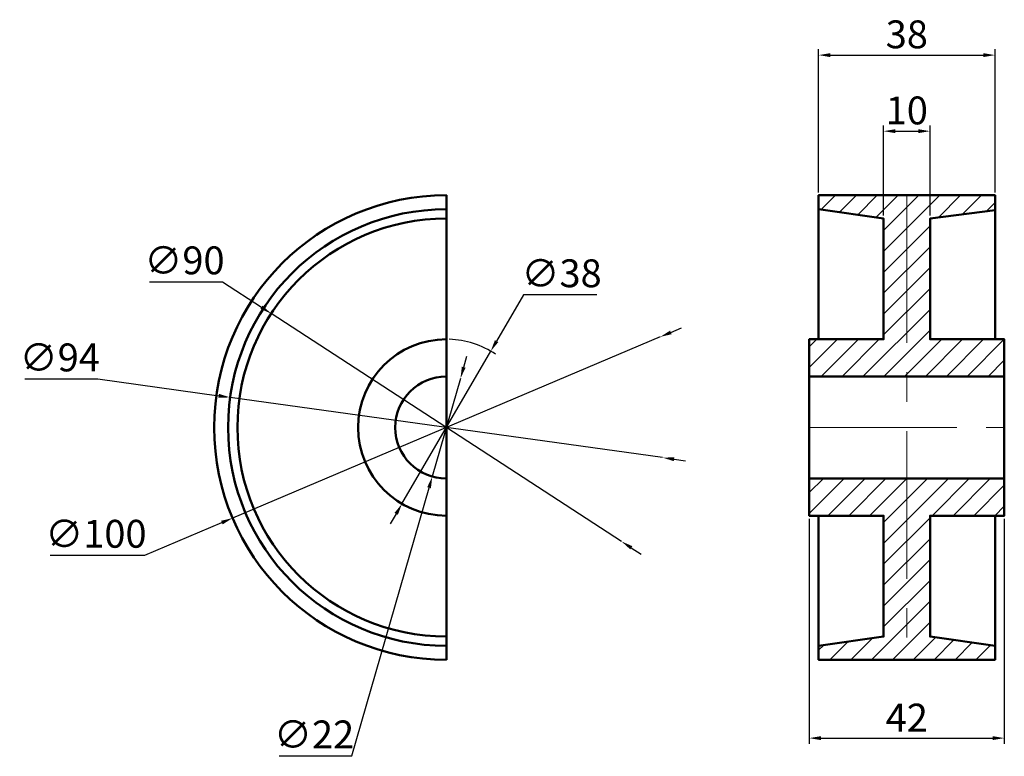
# Model space of a CAD drawing. Units: millimetres. Extents: x 59 to 271, y 50 to 208.
import ezdxf

# ---------------------------------------------------------------- set-up
doc = ezdxf.new("R2010")
doc.units = ezdxf.units.MM
doc.linetypes.add('CENTER', pattern=[50.8, 31.75, -6.35, 6.35, -6.35])
for name, color, linetype, lineweight in [('M-CNTR', 1, 'CENTER', 18), ('M-DIMS', 2, 'Continuous', 25), ('M-HATC', 8, 'Continuous', 18), ('M-OUTL', 7, 'Continuous', 50)]:
    doc.layers.add(name, color=color, linetype=linetype, lineweight=lineweight)
doc.styles.get("Standard").update_dxf_attribs({"font": 'arial.ttf'})
doc.dimstyles.new('ISO-25', dxfattribs={"dimtxt": 6, "dimasz": 2.5, "dimexe": 1.25, "dimexo": 0.625, "dimtad": 1, "dimtoh": 1, "dimdec": 0, "dimtxsty": 'Standard', "dimcen": 2.5, "dimadec": 0, "dimazin": 0, "dimtfac": 1, "dimtdec": 0, "dimtmove": 0, "dimatfit": 3, "dimfxl": 1, "dimarcsym": 0})

# ---------------------------------------------------------------- blocks, each defined once
blk = doc.blocks.new('*D1')
at = {"layer": 'Defpoints', "color": 0, "transparency": 16777216}
for p in [(255.48, 184.43), (245.48, 165.63), (255.48, 165.63)]:
    blk.add_point(p, dxfattribs=at)
at = {"layer": 'M-DIMS', "color": 0, "lineweight": -2, "transparency": 16777216}
for p, q in [((245.48, 166.25), (245.48, 185.68)), ((255.48, 166.25), (255.48, 185.68)), ((247.98, 184.43), (252.98, 184.43))]:
    blk.add_line(p, q, dxfattribs=at)
at = {"layer": 'M-DIMS', "color": 0, "transparency": 16777216}
for points in [[(247.98, 184.85), (247.98, 184.02), (245.48, 184.43)], [(252.98, 184.85), (252.98, 184.02), (255.48, 184.43)]]:
    blk.add_solid(points, dxfattribs=at)
at = {"layer": 'M-DIMS', "color": 0, "transparency": 16777216, "insert": (250.48, 188.12), "char_height": 6, "attachment_point": 5}
blk.add_mtext('10', dxfattribs=at)
blk = doc.blocks.new('*D2')
at = {"layer": 'Defpoints', "color": 0, "transparency": 16777216}
for p in [(269.48, 200.81), (231.48, 170.63), (269.48, 170.63)]:
    blk.add_point(p, dxfattribs=at)
at = {"layer": 'M-DIMS', "color": 0, "lineweight": -2, "transparency": 16777216}
for p, q in [((231.48, 171.25), (231.48, 202.06)), ((269.48, 171.25), (269.48, 202.06)), ((233.98, 200.81), (266.98, 200.81))]:
    blk.add_line(p, q, dxfattribs=at)
at = {"layer": 'M-DIMS', "color": 0, "transparency": 16777216}
for points in [[(233.98, 201.22), (233.98, 200.39), (231.48, 200.81)], [(266.98, 201.22), (266.98, 200.39), (269.48, 200.81)]]:
    blk.add_solid(points, dxfattribs=at)
at = {"layer": 'M-DIMS', "color": 0, "transparency": 16777216, "insert": (250.48, 204.5), "char_height": 6, "attachment_point": 5}
blk.add_mtext('38', dxfattribs=at)
blk = doc.blocks.new('*D3')
at = {"layer": 'Defpoints', "color": 0, "transparency": 16777216}
for p in [(229.48, 101.63), (271.48, 101.63), (271.48, 53.75)]:
    blk.add_point(p, dxfattribs=at)
at = {"layer": 'M-DIMS', "color": 0, "lineweight": -2, "transparency": 16777216}
for p, q in [((229.48, 101), (229.48, 52.5)), ((271.48, 101), (271.48, 52.5)), ((231.98, 53.75), (268.98, 53.75))]:
    blk.add_line(p, q, dxfattribs=at)
at = {"layer": 'M-DIMS', "color": 0, "transparency": 16777216}
for points in [[(231.98, 54.17), (231.98, 53.33), (229.48, 53.75)], [(268.98, 54.17), (268.98, 53.33), (271.48, 53.75)]]:
    blk.add_solid(points, dxfattribs=at)
at = {"layer": 'M-DIMS', "color": 0, "transparency": 16777216, "insert": (250.48, 57.39), "char_height": 6, "attachment_point": 5}
blk.add_mtext('42', dxfattribs=at)
blk = doc.blocks.new('*D4')
at = {"layer": 'Defpoints', "color": 0, "transparency": 16777216}
for p in [(197.37, 140.13), (105.29, 101.13)]:
    blk.add_point(p, dxfattribs=at)
at = {"layer": 'M-DIMS', "color": 0, "lineweight": -2, "transparency": 16777216}
for p, q in [((199.67, 141.1), (201.97, 142.08)), ((197.37, 140.13), (105.29, 101.13)), ((86.37, 93.11), (102.99, 100.15)), ((65.98, 93.11), (86.37, 93.11))]:
    blk.add_line(p, q, dxfattribs=at)
at = {"layer": 'M-DIMS', "color": 0, "transparency": 16777216}
for points in [[(199.51, 141.49), (199.83, 140.72), (197.37, 140.13)], [(102.82, 100.54), (103.15, 99.77), (105.29, 101.13)]]:
    blk.add_solid(points, dxfattribs=at)
at = {"layer": 'M-DIMS', "color": 0, "transparency": 16777216, "insert": (75.86, 96.97), "char_height": 6, "attachment_point": 5}
blk.add_mtext('∅100', dxfattribs=at)
blk = doc.blocks.new('*D5')
at = {"layer": 'Defpoints', "color": 0, "transparency": 16777216}
for p in [(104.78, 127.11), (197.88, 114.14)]:
    blk.add_point(p, dxfattribs=at)
at = {"layer": 'M-DIMS', "color": 0, "lineweight": -2, "transparency": 16777216}
for p, q in [((60.53, 131.08), (76.26, 131.08)), ((76.26, 131.08), (102.3, 127.46)), ((197.88, 114.14), (104.78, 127.11)), ((200.35, 113.8), (202.83, 113.45))]:
    blk.add_line(p, q, dxfattribs=at)
at = {"layer": 'M-DIMS', "color": 0, "transparency": 16777216}
for points in [[(102.36, 127.87), (102.24, 127.04), (104.78, 127.11)], [(200.41, 114.21), (200.3, 113.39), (197.88, 114.14)]]:
    blk.add_solid(points, dxfattribs=at)
at = {"layer": 'M-DIMS', "color": 0, "transparency": 16777216, "insert": (68.08, 134.94), "char_height": 6, "attachment_point": 5}
blk.add_mtext('∅94', dxfattribs=at)
blk = doc.blocks.new('*D6')
at = {"layer": 'Defpoints', "color": 0, "transparency": 16777216}
for p in [(113.6, 145.16), (189.05, 96.1)]:
    blk.add_point(p, dxfattribs=at)
at = {"layer": 'M-DIMS', "color": 0, "lineweight": -2, "transparency": 16777216}
for p, q in [((87.37, 151.99), (103.1, 151.99)), ((103.1, 151.99), (111.51, 146.52)), ((189.05, 96.1), (113.6, 145.16)), ((191.15, 94.73), (193.25, 93.37))]:
    blk.add_line(p, q, dxfattribs=at)
at = {"layer": 'M-DIMS', "color": 0, "transparency": 16777216}
for points in [[(111.73, 146.87), (111.28, 146.17), (113.6, 145.16)], [(191.38, 95.08), (190.92, 94.39), (189.05, 96.1)]]:
    blk.add_solid(points, dxfattribs=at)
at = {"layer": 'M-DIMS', "color": 0, "transparency": 16777216, "insert": (94.93, 155.84), "char_height": 6, "attachment_point": 5}
blk.add_mtext('∅90', dxfattribs=at)
blk = doc.blocks.new('*D7')
at = {"layer": 'Defpoints', "color": 0, "transparency": 16777216}
for p in [(160.88, 137.05), (141.77, 104.2)]:
    blk.add_point(p, dxfattribs=at)
at = {"layer": 'M-DIMS', "color": 0, "lineweight": -2, "transparency": 16777216}
for p, q in [((167.95, 149.2), (162.14, 139.21)), ((183.71, 149.2), (167.95, 149.2)), ((141.77, 104.2), (160.88, 137.05)), ((140.52, 102.04), (139.26, 99.88))]:
    blk.add_line(p, q, dxfattribs=at)
blk.add_arc((151.33, 120.63), 19, 56.0417, 88.1153, dxfattribs=at)
at = {"layer": 'M-DIMS', "color": 0, "transparency": 16777216}
for points in [[(161.78, 139.42), (162.5, 139), (160.88, 137.05)], [(140.16, 102.25), (140.88, 101.83), (141.77, 104.2)]]:
    blk.add_solid(points, dxfattribs=at)
at = {"layer": 'M-DIMS', "color": 0, "transparency": 16777216, "insert": (176.14, 153.06), "char_height": 6, "attachment_point": 5}
blk.add_mtext('∅38', dxfattribs=at)
blk = doc.blocks.new('*D8')
at = {"layer": 'Defpoints', "color": 0, "transparency": 16777216}
for p in [(154.37, 131.2), (148.29, 110.06)]:
    blk.add_point(p, dxfattribs=at)
at = {"layer": 'M-DIMS', "color": 0, "lineweight": -2, "transparency": 16777216}
for p, q in [((155.06, 133.6), (155.75, 136)), ((154.37, 131.2), (148.29, 110.06)), ((130.99, 49.92), (147.6, 107.65)), ((115.31, 49.92), (130.99, 49.92))]:
    blk.add_line(p, q, dxfattribs=at)
at = {"layer": 'M-DIMS', "color": 0, "transparency": 16777216}
for points in [[(154.66, 133.72), (155.46, 133.49), (154.37, 131.2)], [(147.2, 107.77), (148, 107.54), (148.29, 110.06)]]:
    blk.add_solid(points, dxfattribs=at)
at = {"layer": 'M-DIMS', "color": 0, "transparency": 16777216, "insert": (122.84, 53.77), "char_height": 6, "attachment_point": 5}
blk.add_mtext('∅22', dxfattribs=at)

msp = doc.modelspace()

# ---------------------------------------------------------------- hatches: boundary and pattern name
at = {"layer": 'M-HATC'}
h = msp.add_hatch(dxfattribs=at)
h.set_pattern_fill('ANSI31', color=256)
h.set_pattern_definition([(45, (60.016, 0), (-2.245064, 2.245064), [])])
h.paths.add_polyline_path([(250.48, 170.63), (231.48, 170.63), (231.48, 167.63), (245.48, 165.63), (245.48, 139.63), (231.48, 139.63), (229.48, 139.63), (229.48, 131.63), (250.48, 131.63)])
h.paths.add_polyline_path([(271.48, 139.63), (269.48, 139.63), (255.48, 139.63), (255.48, 165.63), (269.48, 167.45), (269.48, 170.63), (250.48, 170.63), (250.48, 131.63), (271.48, 131.63)])
h.paths.add_polyline_path([(271.48, 109.63), (250.48, 109.63), (250.48, 70.63), (269.48, 70.63), (269.48, 73.63), (255.48, 75.63), (255.48, 101.63), (269.48, 101.63), (271.48, 101.63)])
h.paths.add_polyline_path([(250.48, 109.63), (229.48, 109.63), (229.48, 101.63), (231.48, 101.63), (245.48, 101.63), (245.48, 75.63), (231.48, 73.63), (231.48, 70.63), (250.48, 70.63)])

# ---------------------------------------------------------------- linework, layer by layer
at = {"layer": 'M-CNTR'}
for p, q in [((250.48, 170.63), (250.48, 70.63)), ((229.48, 120.63), (271.48, 120.63))]:
    msp.add_line(p, q, dxfattribs=at)
at = {"layer": 'M-OUTL'}
for p, q in [((271.48, 131.63), (229.48, 131.63)), ((229.48, 109.63), (271.48, 109.63))]:
    msp.add_line(p, q, dxfattribs=at)
msp.add_lwpolyline([(151.33, 70.63), (151.33, 170.63, 1)], format="xyb", close=True, dxfattribs=at)
for points in [[(231.48, 139.63), (231.48, 170.63), (269.48, 170.63), (269.48, 139.63)], [(269.48, 73.63), (255.48, 75.63), (255.48, 101.63), (269.48, 101.63), (269.48, 70.63), (231.48, 70.63), (231.48, 101.63), (229.48, 101.63), (229.48, 139.63), (231.48, 139.63), (245.48, 139.63), (245.48, 165.63), (231.48, 167.63)], [(269.48, 101.63), (271.48, 101.63), (271.48, 139.63), (269.48, 139.63), (255.48, 139.63), (255.48, 165.63), (269.48, 167.45)], [(231.48, 73.63), (245.48, 75.63), (245.48, 101.63), (231.48, 101.63)]]:
    msp.add_lwpolyline(points, dxfattribs=at)
for radius in [47, 45, 19, 11]:
    msp.add_arc((151.33, 120.63), radius, 90, 270, dxfattribs=at)

# ---------------------------------------------------------------- dimensions: what is measured, and where the dimension line sits
at = {"layer": 'M-DIMS'}
for base, p1, p2, picture, middle in [((269.48, 200.81), (231.48, 170.63), (269.48, 170.63), '*D2', (250.48, 204.5)), ((255.48, 184.43), (245.48, 165.63), (255.48, 165.63), '*D1', (250.48, 188.12)), ((271.48, 53.75), (229.48, 101.63), (271.48, 101.63), '*D3', (250.48, 57.39))]:
    dim = msp.add_linear_dim(base=base, p1=p1, p2=p2, dimstyle='ISO-25', override={"dimclrd": 0, "dimclre": 0, "dimclrt": 0}, dxfattribs=at)
    dim.commit()
    dim.dimension.update_dxf_attribs({"geometry": picture, "text_midpoint": middle})
for p1, p2, picture, middle in [((189.05, 96.1), (113.6, 145.16), '*D6', (94.93, 151.99)), ((141.77, 104.2), (160.88, 137.05), '*D7', (176.14, 149.2)), ((197.37, 140.13), (105.29, 101.13), '*D4', (75.86, 93.11)), ((197.88, 114.14), (104.78, 127.11), '*D5', (76.26, 131.08)), ((154.37, 131.2), (148.29, 110.06), '*D8', (122.84, 49.92))]:
    dim = msp.add_diameter_dim_2p(p1=p1, p2=p2, dimstyle='ISO-25', override={"dimclrd": 0, "dimclre": 0, "dimclrt": 0}, dxfattribs=at)
    dim.commit()
    dim.dimension.update_dxf_attribs({"geometry": picture, "text_midpoint": middle, "dimtype": 163})

doc.saveas('drawing.dxf')
